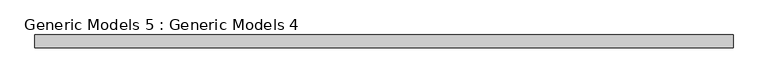
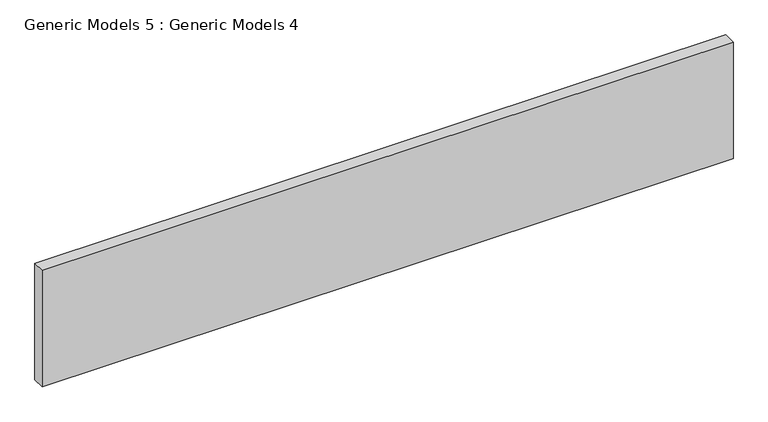
"""IFC4 building model written with IfcOpenShell, lengths in millimetres: proxy geometry, Generic Models 5 : Generic Models 4."""

from ifc_helpers import new_model, si_unit, frame, origin, place, context, project, spatial, polyline, outline, extrude, source, transform, mapped, element, save


def generic_models_5_generic_models_4_8e188f4a(model_context):
    return source(origin(), model_context, "Body", "SweptSolid", [
        extrude(outline(polyline([(497.6218735, -6011.2432543), (-3134.5781265, -6011.2432543), (-3134.5781265, -5944.8090355), (497.6218735, -5944.8090355), (497.6218735, -6011.2432543)])), frame((0.0, 0.0, 5791.2), z_axis=(0.0, 0.0, 1.0), x_axis=(1.0, 0.0, 0.0)), (0.0, 0.0, 1.0), 647.2402172),
    ])


if __name__ == "__main__":
    model = new_model("IFC4")
    model_context = context("Model", 3, world=origin())
    ifc_project = project(units=[si_unit("LENGTHUNIT", "METRE", prefix="MILLI")], contexts=[model_context])
    site = spatial("IfcSite", under=ifc_project)
    building = spatial("IfcBuilding", under=site)
    placement = place(None, origin())
    generic_models_5_generic_models_4_shape = generic_models_5_generic_models_4_8e188f4a(model_context)
    element("IfcBuildingElementProxy", 1, Name="Generic Models 5 : Generic Models 4", ObjectType="Generic Models 5 : Generic Models 4", at=placement, inside=building, context=model_context, shape_type="MappedRepresentation", body=[
        mapped(generic_models_5_generic_models_4_shape, transform((0.0, 0.0, 0.0), x_axis=(1.0, 0.0, 0.0), y_axis=(0.0, 1.0, 0.0), z_axis=(0.0, 0.0, 1.0))),
    ])
    save(model, "model.ifc")
